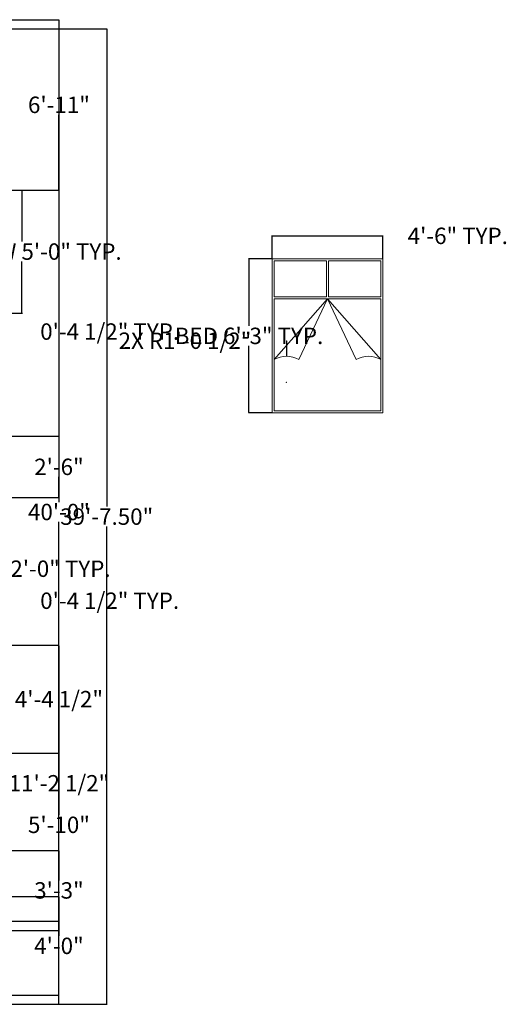
# Model space of a CAD drawing. Units: inches. Extents: x -27 to 662, y -19 to 539.
# Tile 4 of 4: x 425 to 662, y 20 to 500. Entities that reach past the tile are written whole.
import ezdxf

# ---------------------------------------------------------------- set-up
doc = ezdxf.new("R2010")
doc.units = ezdxf.units.IN
doc.header["$MEASUREMENT"] = 0
doc.layers.add('A-ANNO-DIMS', color=2, linetype='Continuous', lineweight=18)
doc.layers.add('A-FURN', color=240, linetype='Continuous', lineweight=18)
doc.styles.get("Standard").update_dxf_attribs({"font": 'italic8.shx'})
doc.dimstyles.get("Standard").update_dxf_attribs({"dimtxt": 8, "dimasz": 0.18, "dimexe": 0.18, "dimexo": 0.0625, "dimgap": 0.09, "dimtad": 0, "dimtih": 1, "dimtoh": 1, "dimzin": 0, "dimdsep": 46, "dimlunit": 3, "dimtxsty": 'Standard', "dimcen": 0.09, "dimclrt": 4, "dimadec": 0, "dimazin": 0, "dimtfac": 1, "dimtofl": 0, "dimtmove": 0, "dimatfit": 3, "dimfxl": 1, "dimtolj": 1, "dimtzin": 0, "dimarcsym": 0})

# ---------------------------------------------------------------- blocks, each defined once
blk = doc.blocks.new('*D2')
at = {"layer": 'A-ANNO-DIMS', "color": 0, "lineweight": -2, "transparency": 16777216}
for p, q in [((391.54, 495.42), (467.74, 495.42)), ((467.56, 495.24), (467.56, 262.52)), ((467.56, 20.1), (467.56, 252.82)), ((391.54, 19.92), (467.74, 19.92))]:
    blk.add_line(p, q, dxfattribs=at)
at = {"layer": 'A-ANNO-DIMS', "color": 0, "transparency": 16777216}
for points in [[(467.53, 495.24), (467.59, 495.24), (467.56, 495.42)], [(467.53, 20.1), (467.59, 20.1), (467.56, 19.92)]]:
    blk.add_solid(points, dxfattribs=at)
at = {"layer": 'Defpoints', "color": 0, "transparency": 16777216}
for p in [(391.48, 495.42), (467.56, 495.42), (391.48, 19.92)]:
    blk.add_point(p, dxfattribs=at)
at = {"layer": 'A-ANNO-DIMS', "color": 0, "transparency": 16777216, "insert": (467.56, 257.67), "char_height": 8, "attachment_point": 5}
blk.add_mtext('\\A1;39\'-7.50"', dxfattribs=at)
blk = doc.blocks.new('BED-DOUBLE-54x75')
for p, q in [((26.5, 56.54), (26.5, 74)), ((27.5, 56.54), (27.5, 74)), ((1, 56.54), (26.5, 56.54)), ((1, 55.54), (53, 55.54)), ((27, 55.54), (1, 26.04)), ((13, 26.04), (27, 55.54)), ((27, 55.54), (53, 26.04)), ((41, 26.04), (27, 55.54)), ((27.5, 56.54), (53, 56.54))]:
    blk.add_line(p, q)
blk.add_lwpolyline([(0, 75), (54, 75), (54, 0), (0, 0)], close=True)
for points in [[(1, 56.54), (1, 74), (26.5, 74)], [(27.5, 74), (53, 74), (53, 56.54)], [(53, 55.54), (53, 1), (1, 1), (1, 55.54)]]:
    blk.add_lwpolyline(points)
for centre in [(7, 14.92), (47, 14.92)]:
    blk.add_arc(centre, 12.64, 61.656, 118.344)
blk = doc.blocks.new('*D12')
at = {"layer": 'A-ANNO-DIMS', "color": 0, "lineweight": -2, "transparency": 16777216}
for p, q in [((548.03, 383.28), (536.66, 383.28)), ((536.84, 383.1), (536.84, 350.64)), ((536.84, 308.46), (536.84, 340.93)), ((548.03, 308.28), (536.66, 308.28))]:
    blk.add_line(p, q, dxfattribs=at)
at = {"layer": 'A-ANNO-DIMS', "color": 0, "transparency": 16777216}
for points in [[(536.81, 383.1), (536.87, 383.1), (536.84, 383.28)], [(536.81, 308.46), (536.87, 308.46), (536.84, 308.28)]]:
    blk.add_solid(points, dxfattribs=at)
at = {"layer": 'Defpoints', "color": 0, "transparency": 16777216}
for p in [(536.84, 383.28), (548.09, 383.28), (548.09, 308.28)]:
    blk.add_point(p, dxfattribs=at)
at = {"layer": 'A-ANNO-DIMS', "color": 4, "transparency": 16777216, "insert": (536.84, 345.78), "char_height": 8, "attachment_point": 5}
blk.add_mtext('\\A1;BED 6\'-3" TYP.', dxfattribs=at)
blk = doc.blocks.new('*D13')
at = {"layer": 'A-ANNO-DIMS', "color": 0, "lineweight": -2, "transparency": 16777216}
for p, q in [((548.09, 383.35), (548.09, 394.71)), ((548.27, 394.53), (601.91, 394.53)), ((602.09, 383.35), (602.09, 394.71)), ((602.09, 394.53), (602.27, 394.53))]:
    blk.add_line(p, q, dxfattribs=at)
at = {"layer": 'A-ANNO-DIMS', "color": 0, "transparency": 16777216}
for points in [[(548.27, 394.56), (548.27, 394.5), (548.09, 394.53)], [(601.91, 394.56), (601.91, 394.5), (602.09, 394.53)]]:
    blk.add_solid(points, dxfattribs=at)
at = {"layer": 'Defpoints', "color": 0, "transparency": 16777216}
for p in [(602.09, 394.53), (548.09, 383.28), (602.09, 383.28)]:
    blk.add_point(p, dxfattribs=at)
at = {"layer": 'A-ANNO-DIMS', "color": 4, "transparency": 16777216, "insert": (638.55, 394.53), "char_height": 8, "attachment_point": 5}
blk.add_mtext('\\A1;4\'-6" TYP.', dxfattribs=at)
blk = doc.blocks.new('*D22')
at = {"layer": 'A-ANNO-DIMS', "color": 0, "lineweight": -2, "transparency": 16777216}
for p, q in [((417.35, 416.88), (426.47, 416.88)), ((426.29, 416.7), (426.29, 391.73)), ((426.29, 357.06), (426.29, 382.03)), ((417.35, 356.88), (426.47, 356.88))]:
    blk.add_line(p, q, dxfattribs=at)
at = {"layer": 'A-ANNO-DIMS', "color": 0, "transparency": 16777216}
for points in [[(426.26, 416.7), (426.32, 416.7), (426.29, 416.88)], [(426.26, 357.06), (426.32, 357.06), (426.29, 356.88)]]:
    blk.add_solid(points, dxfattribs=at)
at = {"layer": 'Defpoints', "color": 0, "transparency": 16777216}
for p in [(417.29, 416.88), (426.29, 416.88), (417.29, 356.88)]:
    blk.add_point(p, dxfattribs=at)
at = {"layer": 'A-ANNO-DIMS', "color": 4, "transparency": 16777216, "insert": (426.29, 386.88), "char_height": 8, "attachment_point": 5}
blk.add_mtext('\\A1;WINDOW 5\'-0" TYP.', dxfattribs=at)
blk = doc.blocks.new('*D23')
at = {"layer": 'A-ANNO-DIMS', "color": 0, "lineweight": -2, "transparency": 16777216}
for p, q in [((412.79, 356.82), (412.79, 347.7)), ((417.29, 356.82), (417.29, 347.7)), ((412.97, 347.88), (417.11, 347.88)), ((417.29, 347.88), (417.47, 347.88))]:
    blk.add_line(p, q, dxfattribs=at)
at = {"layer": 'A-ANNO-DIMS', "color": 0, "transparency": 16777216}
for points in [[(412.97, 347.91), (412.97, 347.85), (412.79, 347.88)], [(417.11, 347.91), (417.11, 347.85), (417.29, 347.88)]]:
    blk.add_solid(points, dxfattribs=at)
at = {"layer": 'Defpoints', "color": 0, "transparency": 16777216}
for p in [(412.79, 356.88), (417.29, 356.88), (417.29, 347.88)]:
    blk.add_point(p, dxfattribs=at)
at = {"layer": 'A-ANNO-DIMS', "color": 4, "transparency": 16777216, "insert": (468.99, 347.88), "char_height": 8, "attachment_point": 5}
blk.add_mtext('\\A1;0\'-4 1/2" TYP.', dxfattribs=at)
blk = doc.blocks.new('*D26')
at = {"layer": 'A-ANNO-DIMS', "color": 0, "lineweight": -2, "transparency": 16777216}
for p, q in [((417.35, 244.27), (421.07, 244.27)), ((420.89, 244.09), (420.89, 237.12)), ((420.89, 220.45), (420.89, 227.42)), ((417.35, 220.27), (421.07, 220.27))]:
    blk.add_line(p, q, dxfattribs=at)
at = {"layer": 'A-ANNO-DIMS', "color": 0, "transparency": 16777216}
for points in [[(420.86, 244.09), (420.92, 244.09), (420.89, 244.27)], [(420.86, 220.45), (420.92, 220.45), (420.89, 220.27)]]:
    blk.add_solid(points, dxfattribs=at)
at = {"layer": 'Defpoints', "color": 0, "transparency": 16777216}
for p in [(417.29, 244.27), (420.89, 244.27), (417.29, 220.27)]:
    blk.add_point(p, dxfattribs=at)
at = {"layer": 'A-ANNO-DIMS', "color": 4, "transparency": 16777216, "insert": (420.89, 232.27), "char_height": 8, "attachment_point": 5}
blk.add_mtext('\\A1;WINDOW 2\'-0" TYP.', dxfattribs=at)
blk = doc.blocks.new('*D27')
at = {"layer": 'A-ANNO-DIMS', "color": 0, "lineweight": -2, "transparency": 16777216}
for p, q in [((412.79, 220.21), (412.79, 216.49)), ((412.97, 216.67), (417.11, 216.67)), ((417.29, 220.21), (417.29, 216.49)), ((417.29, 216.67), (417.47, 216.67))]:
    blk.add_line(p, q, dxfattribs=at)
at = {"layer": 'A-ANNO-DIMS', "color": 0, "transparency": 16777216}
for points in [[(412.97, 216.7), (412.97, 216.64), (412.79, 216.67)], [(417.11, 216.7), (417.11, 216.64), (417.29, 216.67)]]:
    blk.add_solid(points, dxfattribs=at)
at = {"layer": 'Defpoints', "color": 0, "transparency": 16777216}
for p in [(412.79, 220.27), (417.29, 220.27), (417.29, 216.67)]:
    blk.add_point(p, dxfattribs=at)
at = {"layer": 'A-ANNO-DIMS', "color": 4, "transparency": 16777216, "insert": (468.99, 216.67), "char_height": 8, "attachment_point": 5}
blk.add_mtext('\\A1;0\'-4 1/2" TYP.', dxfattribs=at)
blk = doc.blocks.new('*D30')
at = {"layer": 'A-ANNO-DIMS', "color": 0, "lineweight": -2, "transparency": 16777216}
for p, q in [((417.35, 499.92), (444.47, 499.92)), ((444.29, 499.74), (444.29, 264.77)), ((444.29, 20.1), (444.29, 255.07)), ((391.54, 19.92), (444.47, 19.92))]:
    blk.add_line(p, q, dxfattribs=at)
at = {"layer": 'A-ANNO-DIMS', "color": 0, "transparency": 16777216}
for points in [[(444.26, 499.74), (444.32, 499.74), (444.29, 499.92)], [(444.26, 20.1), (444.32, 20.1), (444.29, 19.92)]]:
    blk.add_solid(points, dxfattribs=at)
at = {"layer": 'Defpoints', "color": 0, "transparency": 16777216}
for p in [(417.29, 499.92), (444.29, 499.92), (391.48, 19.92)]:
    blk.add_point(p, dxfattribs=at)
at = {"layer": 'A-ANNO-DIMS', "color": 4, "transparency": 16777216, "insert": (444.29, 259.92), "char_height": 8, "attachment_point": 5}
blk.add_mtext('\\A1;40\'-0"', dxfattribs=at)
blk = doc.blocks.new('*D32')
at = {"layer": 'A-ANNO-DIMS', "color": 0, "lineweight": -2, "transparency": 16777216}
for p, q in [((270.35, 142.42), (444.47, 142.42)), ((444.29, 142.24), (444.29, 112.27)), ((444.29, 72.6), (444.29, 102.57)), ((270.35, 72.42), (444.47, 72.42))]:
    blk.add_line(p, q, dxfattribs=at)
at = {"layer": 'A-ANNO-DIMS', "color": 0, "transparency": 16777216}
for points in [[(444.26, 142.24), (444.32, 142.24), (444.29, 142.42)], [(444.26, 72.6), (444.32, 72.6), (444.29, 72.42)]]:
    blk.add_solid(points, dxfattribs=at)
at = {"layer": 'Defpoints', "color": 0, "transparency": 16777216}
for p in [(270.29, 142.42), (444.29, 142.42), (270.29, 72.42)]:
    blk.add_point(p, dxfattribs=at)
at = {"layer": 'A-ANNO-DIMS', "color": 4, "transparency": 16777216, "insert": (444.29, 107.42), "char_height": 8, "attachment_point": 5}
blk.add_mtext('\\A1;5\'-10"', dxfattribs=at)
blk = doc.blocks.new('*D33')
at = {"layer": 'A-ANNO-DIMS', "color": 0, "lineweight": -2, "transparency": 16777216}
for p, q in [((270.35, 194.92), (444.47, 194.92)), ((444.29, 194.74), (444.29, 174.85)), ((444.29, 142.6), (444.29, 162.48)), ((270.35, 142.42), (444.47, 142.42))]:
    blk.add_line(p, q, dxfattribs=at)
at = {"layer": 'A-ANNO-DIMS', "color": 0, "transparency": 16777216}
for points in [[(444.26, 194.74), (444.32, 194.74), (444.29, 194.92)], [(444.26, 142.6), (444.32, 142.6), (444.29, 142.42)]]:
    blk.add_solid(points, dxfattribs=at)
at = {"layer": 'Defpoints', "color": 0, "transparency": 16777216}
for p in [(270.29, 194.92), (444.29, 194.92), (270.29, 142.42)]:
    blk.add_point(p, dxfattribs=at)
at = {"layer": 'A-ANNO-DIMS', "color": 4, "transparency": 16777216, "insert": (444.29, 168.67), "char_height": 8, "attachment_point": 5}
blk.add_mtext('\\A1;4\'-4 1/2"', dxfattribs=at)
blk = doc.blocks.new('*D34')
at = {"layer": 'A-ANNO-DIMS', "color": 0, "lineweight": -2, "transparency": 16777216}
for p, q in [((270.35, 72.42), (444.47, 72.42)), ((444.29, 72.24), (444.29, 53.27)), ((444.29, 24.6), (444.29, 43.57)), ((270.35, 24.42), (444.47, 24.42))]:
    blk.add_line(p, q, dxfattribs=at)
at = {"layer": 'A-ANNO-DIMS', "color": 0, "transparency": 16777216}
for points in [[(444.26, 72.24), (444.32, 72.24), (444.29, 72.42)], [(444.26, 24.6), (444.32, 24.6), (444.29, 24.42)]]:
    blk.add_solid(points, dxfattribs=at)
at = {"layer": 'Defpoints', "color": 0, "transparency": 16777216}
for p in [(270.29, 72.42), (444.29, 72.42), (270.29, 24.42)]:
    blk.add_point(p, dxfattribs=at)
at = {"layer": 'A-ANNO-DIMS', "color": 4, "transparency": 16777216, "insert": (444.29, 48.42), "char_height": 8, "attachment_point": 5}
blk.add_mtext('\\A1;4\'-0"', dxfattribs=at)
blk = doc.blocks.new('*D40')
at = {"layer": 'A-ANNO-DIMS', "color": 0, "lineweight": -2, "transparency": 16777216}
for p, q in [((412.85, 194.92), (444.47, 194.92)), ((444.29, 194.74), (444.29, 133.85)), ((444.29, 60.6), (444.29, 121.48)), ((412.85, 60.42), (444.47, 60.42))]:
    blk.add_line(p, q, dxfattribs=at)
at = {"layer": 'A-ANNO-DIMS', "color": 0, "transparency": 16777216}
for points in [[(444.26, 194.74), (444.32, 194.74), (444.29, 194.92)], [(444.26, 60.6), (444.32, 60.6), (444.29, 60.42)]]:
    blk.add_solid(points, dxfattribs=at)
at = {"layer": 'Defpoints', "color": 0, "transparency": 16777216}
for p in [(412.79, 194.92), (444.29, 194.92), (412.79, 60.42)]:
    blk.add_point(p, dxfattribs=at)
at = {"layer": 'A-ANNO-DIMS', "color": 4, "transparency": 16777216, "insert": (444.29, 127.67), "char_height": 8, "attachment_point": 5}
blk.add_mtext('\\A1;11\'-2 1/2"', dxfattribs=at)
blk = doc.blocks.new('*D50')
at = {"layer": 'A-ANNO-DIMS', "color": 0, "lineweight": -2, "transparency": 16777216}
for p, q in [((417.35, 499.92), (444.47, 499.92)), ((444.29, 499.74), (444.29, 463.25)), ((444.29, 417.06), (444.29, 453.55)), ((417.35, 416.88), (444.47, 416.88))]:
    blk.add_line(p, q, dxfattribs=at)
at = {"layer": 'A-ANNO-DIMS', "color": 0, "transparency": 16777216}
for points in [[(444.26, 499.74), (444.32, 499.74), (444.29, 499.92)], [(444.26, 417.06), (444.32, 417.06), (444.29, 416.88)]]:
    blk.add_solid(points, dxfattribs=at)
at = {"layer": 'Defpoints', "color": 0, "transparency": 16777216}
for p in [(417.29, 499.92), (444.29, 499.92), (417.29, 416.88)]:
    blk.add_point(p, dxfattribs=at)
at = {"layer": 'A-ANNO-DIMS', "color": 4, "transparency": 16777216, "insert": (444.29, 458.4), "char_height": 8, "attachment_point": 5}
blk.add_mtext('\\A1;6\'-11"', dxfattribs=at)
blk = doc.blocks.new('*D51')
at = {"layer": 'A-ANNO-DIMS', "color": 0, "lineweight": -2, "transparency": 16777216}
for p, q in [((417.35, 94.96), (444.47, 94.96)), ((444.29, 94.78), (444.29, 80.29)), ((444.29, 56.1), (444.29, 70.59)), ((417.35, 55.92), (444.47, 55.92))]:
    blk.add_line(p, q, dxfattribs=at)
at = {"layer": 'A-ANNO-DIMS', "color": 0, "transparency": 16777216}
for points in [[(444.26, 94.78), (444.32, 94.78), (444.29, 94.96)], [(444.26, 56.1), (444.32, 56.1), (444.29, 55.92)]]:
    blk.add_solid(points, dxfattribs=at)
at = {"layer": 'Defpoints', "color": 0, "transparency": 16777216}
for p in [(417.29, 94.96), (444.29, 94.96), (417.29, 55.92)]:
    blk.add_point(p, dxfattribs=at)
at = {"layer": 'A-ANNO-DIMS', "color": 4, "transparency": 16777216, "insert": (444.29, 75.44), "char_height": 8, "attachment_point": 5}
blk.add_mtext('\\A1;3\'-3"', dxfattribs=at)
blk = doc.blocks.new('*D53')
at = {"layer": 'A-ANNO-DIMS', "color": 0, "lineweight": -2, "transparency": 16777216}
for p, q in [((109.35, 296.92), (444.47, 296.92)), ((444.29, 296.74), (444.29, 286.77)), ((444.29, 267.1), (444.29, 277.07)), ((109.35, 266.92), (444.47, 266.92))]:
    blk.add_line(p, q, dxfattribs=at)
at = {"layer": 'A-ANNO-DIMS', "color": 0, "transparency": 16777216}
for points in [[(444.26, 296.74), (444.32, 296.74), (444.29, 296.92)], [(444.26, 267.1), (444.32, 267.1), (444.29, 266.92)]]:
    blk.add_solid(points, dxfattribs=at)
at = {"layer": 'Defpoints', "color": 0, "transparency": 16777216}
for p in [(109.29, 296.92), (444.29, 296.92), (109.29, 266.92)]:
    blk.add_point(p, dxfattribs=at)
at = {"layer": 'A-ANNO-DIMS', "color": 4, "transparency": 16777216, "insert": (444.29, 281.92), "char_height": 8, "attachment_point": 5}
blk.add_mtext('\\A1;2\'-6"', dxfattribs=at)
blk = doc.blocks.new('*D59')
at = {"layer": 'A-ANNO-DIMS', "color": 0, "lineweight": -2, "transparency": 16777216}
for p, q in [((554.91, 343.42), (555.09, 343.42)), ((555.09, 343.42), (555.09, 336.02)), ((555, 323.2), (555.18, 323.2)), ((555.09, 323.11), (555.09, 323.29))]:
    blk.add_line(p, q, dxfattribs=at)
at = {"layer": 'A-ANNO-DIMS', "color": 0, "transparency": 16777216}
blk.add_solid([(555.12, 336.02), (555.06, 336.02), (555.09, 335.84)], dxfattribs=at)
at = {"layer": 'Defpoints', "color": 0, "transparency": 16777216}
for p in [(555.09, 335.84), (555.09, 323.2)]:
    blk.add_point(p, dxfattribs=at)
at = {"layer": 'A-ANNO-DIMS', "color": 4, "transparency": 16777216, "insert": (505.67, 343.42), "char_height": 8, "attachment_point": 5}
blk.add_mtext('\\A1;2X R1\'-0 1/2"', dxfattribs=at)

msp = doc.modelspace()

# ---------------------------------------------------------------- block references
at = {"layer": 'A-FURN'}
msp.add_blockref('BED-DOUBLE-54x75', (548.088, 308.283), dxfattribs=at)

# ---------------------------------------------------------------- dimensions: what is measured, and where the dimension line sits
at = {"layer": 'A-ANNO-DIMS'}
for base, p1, p2, override, picture, middle in [((444.288, 499.919), (391.48, 19.919), (417.288, 499.919), {"dimdec": 1, "dimlfac": 1, "dimrnd": 0, "dimzin": 1, "dimdsep": 46, "dimlunit": 4, "dimfrac": 2}, '*D30', (444.288, 259.919)), ((444.288, 499.919), (417.288, 416.883), (417.288, 499.919), {"dimdec": 1, "dimlfac": 1, "dimrnd": 0, "dimzin": 1, "dimdsep": 46, "dimlunit": 4, "dimfrac": 2}, '*D50', (444.288, 458.401)), ((467.557, 495.419), (391.48, 19.919), (391.48, 495.419), {"dimclrd": 0, "dimclre": 0, "dimclrt": 0}, '*D2', (467.557, 257.669)), ((444.288, 296.919), (109.288, 266.919), (109.288, 296.919), {"dimdec": 1, "dimlfac": 1, "dimrnd": 0, "dimzin": 1, "dimdsep": 46, "dimlunit": 4, "dimfrac": 2}, '*D53', (444.288, 281.919)), ((444.288, 194.919), (270.288, 142.419), (270.288, 194.919), {"dimdec": 1, "dimlfac": 1, "dimrnd": 0, "dimzin": 1, "dimdsep": 46, "dimlunit": 4, "dimfrac": 2}, '*D33', (444.288, 168.669)), ((444.288, 194.919), (412.788, 60.419), (412.788, 194.919), {"dimdec": 1, "dimlfac": 1, "dimrnd": 0, "dimzin": 1, "dimdsep": 46, "dimlunit": 4, "dimfrac": 2}, '*D40', (444.288, 127.669)), ((444.288, 142.419), (270.288, 72.419), (270.288, 142.419), {"dimdec": 1, "dimlfac": 1, "dimrnd": 0, "dimzin": 1, "dimdsep": 46, "dimlunit": 4, "dimfrac": 2}, '*D32', (444.288, 107.419)), ((444.288, 94.965), (417.288, 55.919), (417.288, 94.965), {"dimdec": 1, "dimlfac": 1, "dimrnd": 0, "dimzin": 1, "dimdsep": 46, "dimlunit": 4, "dimfrac": 2}, '*D51', (444.288, 75.442)), ((444.288, 72.419), (270.288, 24.419), (270.288, 72.419), {"dimdec": 1, "dimlfac": 1, "dimrnd": 0, "dimzin": 1, "dimdsep": 46, "dimlunit": 4, "dimfrac": 2}, '*D34', (444.288, 48.419))]:
    dim = msp.add_linear_dim(base=base, p1=p1, p2=p2, angle=90, dimstyle='Standard', override=override, dxfattribs=at)
    dim.commit()
    dim.dimension.update_dxf_attribs({"geometry": picture, "text_midpoint": middle})
for base, p1, p2, text, picture, middle in [((426.288, 416.883), (417.288, 356.883), (417.288, 416.883), 'WINDOW <> TYP.', '*D22', (426.288, 386.883)), ((536.838, 383.283), (548.088, 308.283), (548.088, 383.283), 'BED <> TYP.', '*D12', (536.838, 345.783)), ((420.888, 244.271), (417.288, 220.271), (417.288, 244.271), 'WINDOW <> TYP.', '*D26', (420.888, 232.271))]:
    dim = msp.add_linear_dim(base=base, p1=p1, p2=p2, angle=90, text=text, dimstyle='Standard', override={"dimdec": 1, "dimlfac": 1, "dimrnd": 0, "dimzin": 1, "dimdsep": 46, "dimlunit": 4, "dimfrac": 2}, dxfattribs=at)
    dim.commit()
    dim.dimension.update_dxf_attribs({"geometry": picture, "text_midpoint": middle})
for base, p1, p2, picture, middle in [((602.088, 394.533), (548.088, 383.283), (602.088, 383.283), '*D13', (638.549, 394.533)), ((417.288, 347.883), (412.788, 356.883), (417.288, 356.883), '*D23', (468.986, 347.883)), ((417.288, 216.671), (412.788, 220.271), (417.288, 220.271), '*D27', (468.986, 216.671))]:
    dim = msp.add_linear_dim(base=base, p1=p1, p2=p2, text='<> TYP.', dimstyle='Standard', override={"dimdec": 1, "dimlfac": 1, "dimrnd": 0, "dimzin": 1, "dimdsep": 46, "dimlunit": 4, "dimfrac": 2}, dxfattribs=at)
    dim.commit()
    dim.dimension.update_dxf_attribs({"geometry": picture, "text_midpoint": middle})
dim = msp.add_radius_dim(center=(555.088, 323.2), mpoint=(555.088, 335.837), text='2X <>', dimstyle='Standard', override={"dimdec": 1, "dimlfac": 1, "dimrnd": 0, "dimzin": 1, "dimdsep": 46, "dimlunit": 4, "dimfrac": 2}, dxfattribs=at)
dim.commit()
dim.dimension.update_dxf_attribs({"geometry": '*D59', "text_midpoint": (505.675, 343.42), "dimtype": 164})

doc.saveas('drawing.dxf')
